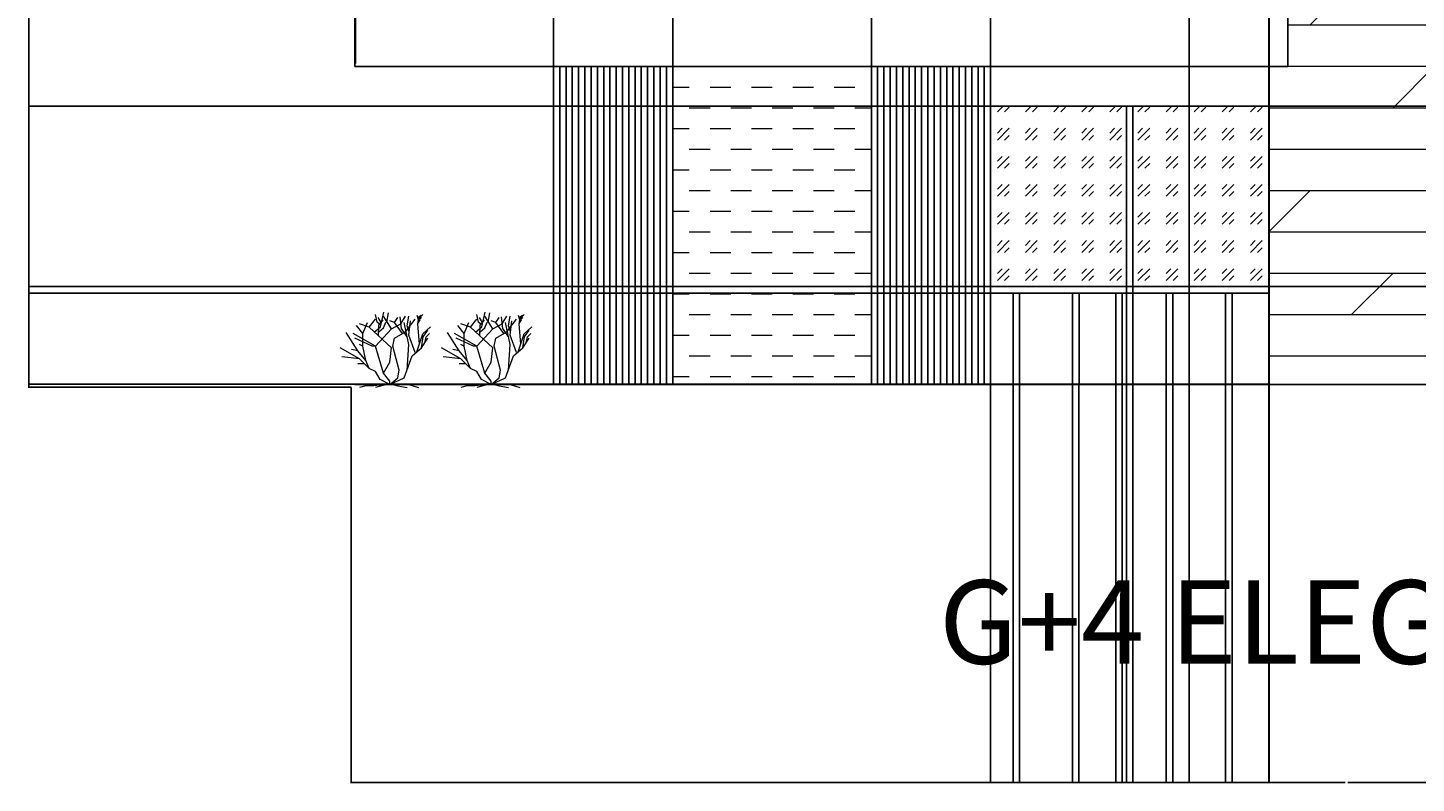
# Model space of a CAD drawing. Units: inches. Extents: x 250 to 1217, y -42 to 832.
# Tile 1 of 7: x 250 to 670, y -42 to 187. Entities that reach past the tile are written whole.
import ezdxf

# ---------------------------------------------------------------- set-up
doc = ezdxf.new("R2010")
doc.units = ezdxf.units.IN
doc.header["$MEASUREMENT"] = 0
for name, color, linetype, lineweight in [('A-ANNO-DIMS', 2, 'Continuous', 18), ('A-ANNO-TEXT', 7, 'Continuous', 25), ('A-ELEV', 7, 'Continuous', 25), ('A-ELEV-PATT', 8, 'Continuous', 13), ('L-PLNT', 3, 'Continuous', 13)]:
    doc.layers.add(name, color=color, linetype=linetype, lineweight=lineweight)
doc.styles.get("Standard").update_dxf_attribs({"font": 'arial.ttf'})
doc.dimstyles.get("Standard").update_dxf_attribs({"dimtxt": 0.18, "dimasz": 0.18, "dimexe": 0.18, "dimexo": 0.0625, "dimgap": 0.09, "dimtad": 0, "dimtih": 1, "dimtoh": 1, "dimdec": 4, "dimzin": 0, "dimdsep": 46, "dimtxsty": 'Standard', "dimcen": 0.09, "dimadec": 0, "dimazin": 0, "dimtfac": 1, "dimtdec": 4, "dimtofl": 0, "dimtmove": 0, "dimatfit": 3, "dimfxl": 1, "dimtolj": 1, "dimtzin": 0, "dimarcsym": 0})

# ---------------------------------------------------------------- blocks, each defined once
blk = doc.blocks.new('*U2')
for p, q in [((-12.471, 19.775), (-12.898, 22.044)), ((-11.28, 19.619), (-12.104, 21.184)), ((-11.433, 18.289), (-10.457, 22.749)), ((-8.16, 17.76), (-10.56, 21.6)), ((-9.48, 19.775), (-8.992, 22.592)), ((-7.2, 19.68), (-6.24, 21.12)), ((-5.086, 17.741), (-5.513, 21.34)), ((-5.28, 19.2), (-3.84, 21.6)), ((-3.377, 18.602), (-2.888, 21.575)), ((-0.508, 21.888), (-0.081, 20.558)), ((-0.203, 19.149), (0.102, 21.34)), ((-0.02, 20.01), (0.896, 21.105)), ((0.041, 20.714), (1.384, 22.044)), ((0.102, 21.34), (0.835, 21.888)), ((-16.8, 16.32), (-18.72, 18.72)), ((-14.88, 18.24), (-17.76, 19.2)), ((-16.8, 16.32), (-15.36, 19.68)), ((-14.88, 18.24), (-12.96, 20.64)), ((-8.16, 12), (-14.88, 18.24)), ((-13.325, 16.724), (-11.433, 18.289)), ((-12.96, 12.48), (-8.16, 17.76)), ((-11.677, 19.071), (-12.471, 19.775)), ((-12.043, 15.628), (-11.921, 18.836)), ((-11.982, 16.802), (-10.579, 18.054)), ((-11.921, 18.836), (-10.64, 20.401)), ((-10.579, 18.054), (-9.846, 19.697)), ((-7.2, 19.68), (-8.64, 20.16)), ((-8.16, 17.76), (-5.28, 19.2)), ((-4.8, 16.32), (-7.2, 19.68)), ((-7.2, 14.88), (-3.84, 16.8)), ((-3.377, 15.315), (-5.086, 17.819)), ((-2.88, 12.96), (-4.32, 19.68)), ((-3.84, 16.8), (-0.96, 20.64)), ((-2.766, 16.802), (-3.377, 18.602)), ((-2.88, 15.84), (-2.4, 20.16)), ((0.346, 13.203), (-0.203, 19.149)), ((-0.142, 19.384), (0.59, 20.401)), ((1.323, 16.254), (3.642, 18.289)), ((1.44, 15.36), (2.88, 17.28)), ((-18.24, 11.04), (-21.755, 16.655)), ((-12.96, 12.48), (-19.68, 16.32)), ((-13.92, 12.48), (-19.2, 14.88)), ((-16.8, 12.48), (-17.76, 12.96)), ((-16.8, 12.48), (-16.8, 16.32)), ((-7.68, 12.48), (-7.2, 14.88)), ((-3.36, 5.28), (-2.88, 12.96)), ((-0.96, 10.56), (-2.88, 15.84)), ((-0.48, 10.8), (0.346, 13.203)), ((0.346, 13.203), (1.323, 16.254)), ((0.96, 12), (1.44, 15.36)), ((0.96, 12), (2.88, 14.88)), ((1.92, 13.44), (2.4, 15.36)), ((2.4, 15.36), (3.36, 16.32)), ((-17.76, 8.64), (-23.663, 11.961)), ((-17.76, 8.64), (-23.128, 9.222)), ((-18.24, 11.04), (-20.16, 11.52)), ((-15.84, 8.16), (-18.24, 11.04)), ((-14.88, 5.76), (-17.76, 8.64)), ((-15.84, 8.16), (-16.8, 12.48)), ((-12.96, 12.48), (-13.92, 12.48)), ((-10.56, 4.32), (-12.96, 12.48)), ((-8.64, 7.68), (-8.16, 12)), ((-6.72, 8.64), (-7.68, 12.48)), ((-5.76, 5.28), (-6.72, 8.64)), ((-4.32, 2.88), (-1.92, 9.6)), ((-1.92, 9.6), (0.96, 12)), ((-16.32, 7.2), (-18.24, 7.2)), ((-14.88, 5.76), (-15.84, 8.16)), ((-12.96, 4.8), (-14.88, 5.76)), ((-11.52, 2.4), (-12.96, 4.8)), ((-10.56, 4.32), (-8.64, 7.68)), ((-8.64, 1.92), (-10.56, 4.32)), ((-6.24, 2.88), (-5.76, 5.28)), ((-15.84, 0.48), (-17.76, 0)), ((-13.44, 0.48), (-15.84, 0.48)), ((-9.6, 0.96), (-13.44, 0.48)), ((-9.6, 0.96), (-12.96, 0)), ((-8.64, 0.96), (-11.52, 2.4)), ((-9.6, 0.96), (-7.68, 0.96)), ((-8.64, 0.96), (-4.32, 2.88)), ((-8.64, 0.96), (-6.24, 2.88)), ((-8.64, 0.96), (-8.64, 1.92)), ((-8.64, 0.96), (-2.88, 0.96)), ((-7.68, 0.96), (-6.24, 0.48)), ((-6.24, 0.48), (-3.36, 0)), ((-2.88, 0.96), (0, 0))]:
    blk.add_line(p, q)
blk = doc.blocks.new('*D7')
at = {"layer": 'A-ANNO-DIMS', "color": 0, "lineweight": -2, "transparency": 16777216}
for p, q in [((347.9, 78), (347.9, -41.6)), ((948.98, 78.86), (948.98, -41.6)), ((348.08, -41.42), (648.06, -41.42)), ((948.8, -41.42), (648.82, -41.42))]:
    blk.add_line(p, q, dxfattribs=at)
at = {"layer": 'A-ANNO-DIMS', "color": 0, "transparency": 16777216}
for points in [[(348.08, -41.39), (348.08, -41.45), (347.9, -41.42)], [(948.8, -41.39), (948.8, -41.45), (948.98, -41.42)]]:
    blk.add_solid(points, dxfattribs=at)
at = {"layer": 'Defpoints', "color": 0, "transparency": 16777216}
for p in [(347.9, 78.06), (948.98, 78.93), (948.98, -41.42)]:
    blk.add_point(p, dxfattribs=at)
at = {"layer": 'A-ANNO-DIMS', "color": 0, "transparency": 16777216, "insert": (648.44, -41.42), "char_height": 0.18, "attachment_point": 5}
blk.add_mtext('\\A1;601.1', dxfattribs=at)
blk = doc.blocks.new('*D11')
at = {"layer": 'A-ANNO-DIMS', "color": 0, "lineweight": -2, "transparency": 16777216}
for p, q in [((352.28, 702.93), (250.36, 702.93)), ((250.54, 702.75), (250.54, 390.68)), ((250.54, 78.24), (250.54, 390.31)), ((347.84, 78.06), (250.36, 78.06))]:
    blk.add_line(p, q, dxfattribs=at)
at = {"layer": 'A-ANNO-DIMS', "color": 0, "transparency": 16777216}
for points in [[(250.51, 702.75), (250.57, 702.75), (250.54, 702.93)], [(250.51, 78.24), (250.57, 78.24), (250.54, 78.06)]]:
    blk.add_solid(points, dxfattribs=at)
at = {"layer": 'Defpoints', "color": 0, "transparency": 16777216}
for p in [(250.54, 702.93), (352.34, 702.93), (347.9, 78.06)]:
    blk.add_point(p, dxfattribs=at)
at = {"layer": 'A-ANNO-DIMS', "color": 0, "transparency": 16777216, "insert": (250.54, 390.49), "char_height": 0.18, "attachment_point": 5}
blk.add_mtext('\\A1;624.9', dxfattribs=at)
blk = doc.blocks.new('*D22')
at = {"layer": 'A-ANNO-DIMS', "color": 0, "lineweight": -2, "transparency": 16777216}
for p, q in [((349.2, 175.91), (349.2, 831.77)), ((349.38, 831.59), (378.7, 831.59)), ((408.8, 831.59), (379.49, 831.59)), ((408.98, 174.99), (408.98, 831.77))]:
    blk.add_line(p, q, dxfattribs=at)
at = {"layer": 'A-ANNO-DIMS', "color": 0, "transparency": 16777216}
for points in [[(349.38, 831.62), (349.38, 831.56), (349.2, 831.59)], [(408.8, 831.62), (408.8, 831.56), (408.98, 831.59)]]:
    blk.add_solid(points, dxfattribs=at)
at = {"layer": 'Defpoints', "color": 0, "transparency": 16777216}
for p in [(408.98, 831.59), (349.2, 175.84), (408.98, 174.93)]:
    blk.add_point(p, dxfattribs=at)
at = {"layer": 'A-ANNO-DIMS', "color": 0, "transparency": 16777216, "insert": (379.09, 831.59), "char_height": 0.18, "attachment_point": 5}
blk.add_mtext('\\A1;59.78', dxfattribs=at)
blk = doc.blocks.new('*D23')
at = {"layer": 'A-ANNO-DIMS', "color": 0, "lineweight": -2, "transparency": 16777216}
for p, q in [((408.98, 174.99), (408.98, 831.77)), ((409.16, 831.59), (426.76, 831.59)), ((444.8, 831.59), (427.2, 831.59)), ((444.98, 174.99), (444.98, 831.77))]:
    blk.add_line(p, q, dxfattribs=at)
at = {"layer": 'A-ANNO-DIMS', "color": 0, "transparency": 16777216}
for points in [[(409.16, 831.62), (409.16, 831.56), (408.98, 831.59)], [(444.8, 831.62), (444.8, 831.56), (444.98, 831.59)]]:
    blk.add_solid(points, dxfattribs=at)
at = {"layer": 'Defpoints', "color": 0, "transparency": 16777216}
for p in [(444.98, 831.59), (408.98, 174.93), (444.98, 174.93)]:
    blk.add_point(p, dxfattribs=at)
at = {"layer": 'A-ANNO-DIMS', "color": 0, "transparency": 16777216, "insert": (426.98, 831.59), "char_height": 0.18, "attachment_point": 5}
blk.add_mtext('\\A1;36', dxfattribs=at)
blk = doc.blocks.new('*D24')
at = {"layer": 'A-ANNO-DIMS', "color": 0, "lineweight": -2, "transparency": 16777216}
for p, q in [((444.98, 174.99), (444.98, 831.77)), ((445.16, 831.59), (474.76, 831.59)), ((504.8, 831.59), (475.2, 831.59)), ((504.98, 174.99), (504.98, 831.77))]:
    blk.add_line(p, q, dxfattribs=at)
at = {"layer": 'A-ANNO-DIMS', "color": 0, "transparency": 16777216}
for points in [[(445.16, 831.62), (445.16, 831.56), (444.98, 831.59)], [(504.8, 831.62), (504.8, 831.56), (504.98, 831.59)]]:
    blk.add_solid(points, dxfattribs=at)
at = {"layer": 'Defpoints', "color": 0, "transparency": 16777216}
for p in [(504.98, 831.59), (444.98, 174.93), (504.98, 174.93)]:
    blk.add_point(p, dxfattribs=at)
at = {"layer": 'A-ANNO-DIMS', "color": 0, "transparency": 16777216, "insert": (474.98, 831.59), "char_height": 0.18, "attachment_point": 5}
blk.add_mtext('\\A1;60', dxfattribs=at)
blk = doc.blocks.new('*D25')
at = {"layer": 'A-ANNO-DIMS', "color": 0, "lineweight": -2, "transparency": 16777216}
for p, q in [((504.98, 174.99), (504.98, 831.77)), ((505.16, 831.59), (522.76, 831.59)), ((540.8, 831.59), (523.2, 831.59)), ((540.98, 174.99), (540.98, 831.77))]:
    blk.add_line(p, q, dxfattribs=at)
at = {"layer": 'A-ANNO-DIMS', "color": 0, "transparency": 16777216}
for points in [[(505.16, 831.62), (505.16, 831.56), (504.98, 831.59)], [(540.8, 831.62), (540.8, 831.56), (540.98, 831.59)]]:
    blk.add_solid(points, dxfattribs=at)
at = {"layer": 'Defpoints', "color": 0, "transparency": 16777216}
for p in [(540.98, 831.59), (504.98, 174.93), (540.98, 174.93)]:
    blk.add_point(p, dxfattribs=at)
at = {"layer": 'A-ANNO-DIMS', "color": 0, "transparency": 16777216, "insert": (522.98, 831.59), "char_height": 0.18, "attachment_point": 5}
blk.add_mtext('\\A1;36', dxfattribs=at)
blk = doc.blocks.new('*D26')
at = {"layer": 'A-ANNO-DIMS', "color": 0, "lineweight": -2, "transparency": 16777216}
for p, q in [((540.98, 174.99), (540.98, 831.77)), ((541.16, 831.59), (582.76, 831.59)), ((624.8, 831.59), (583.2, 831.59)), ((624.98, 174.99), (624.98, 831.77))]:
    blk.add_line(p, q, dxfattribs=at)
at = {"layer": 'A-ANNO-DIMS', "color": 0, "transparency": 16777216}
for points in [[(541.16, 831.62), (541.16, 831.56), (540.98, 831.59)], [(624.8, 831.62), (624.8, 831.56), (624.98, 831.59)]]:
    blk.add_solid(points, dxfattribs=at)
at = {"layer": 'Defpoints', "color": 0, "transparency": 16777216}
for p in [(624.98, 831.59), (540.98, 174.93), (624.98, 174.93)]:
    blk.add_point(p, dxfattribs=at)
at = {"layer": 'A-ANNO-DIMS', "color": 0, "transparency": 16777216, "insert": (582.98, 831.59), "char_height": 0.18, "attachment_point": 5}
blk.add_mtext('\\A1;84', dxfattribs=at)
blk = doc.blocks.new('*D27')
at = {"layer": 'A-ANNO-DIMS', "color": 0, "lineweight": -2, "transparency": 16777216}
for p, q in [((624.98, 174.99), (624.98, 831.77)), ((625.16, 831.59), (655.07, 831.59)), ((685.76, 831.59), (655.86, 831.59)), ((685.94, 176.49), (685.94, 831.77))]:
    blk.add_line(p, q, dxfattribs=at)
at = {"layer": 'A-ANNO-DIMS', "color": 0, "transparency": 16777216}
for points in [[(625.16, 831.62), (625.16, 831.56), (624.98, 831.59)], [(685.76, 831.62), (685.76, 831.56), (685.94, 831.59)]]:
    blk.add_solid(points, dxfattribs=at)
at = {"layer": 'Defpoints', "color": 0, "transparency": 16777216}
for p in [(685.94, 831.59), (685.94, 176.43), (624.98, 174.93)]:
    blk.add_point(p, dxfattribs=at)
at = {"layer": 'A-ANNO-DIMS', "color": 0, "transparency": 16777216, "insert": (655.46, 831.59), "char_height": 0.18, "attachment_point": 5}
blk.add_mtext('\\A1;60.96', dxfattribs=at)
blk = doc.blocks.new('*D35')
at = {"layer": 'A-ANNO-DIMS', "color": 0, "lineweight": -2, "transparency": 16777216}
for p, q in [((624.92, 106.47), (250.36, 106.47)), ((250.54, 106.29), (250.54, 92.88)), ((250.54, 79.11), (250.54, 92.51)), ((624.92, 78.93), (250.36, 78.93))]:
    blk.add_line(p, q, dxfattribs=at)
at = {"layer": 'A-ANNO-DIMS', "color": 0, "transparency": 16777216}
for points in [[(250.51, 106.29), (250.57, 106.29), (250.54, 106.47)], [(250.51, 79.11), (250.57, 79.11), (250.54, 78.93)]]:
    blk.add_solid(points, dxfattribs=at)
at = {"layer": 'Defpoints', "color": 0, "transparency": 16777216}
for p in [(250.54, 106.47), (624.98, 106.47), (624.98, 78.93)]:
    blk.add_point(p, dxfattribs=at)
at = {"layer": 'A-ANNO-DIMS', "color": 0, "transparency": 16777216, "insert": (250.54, 92.7), "char_height": 0.18, "attachment_point": 5}
blk.add_mtext('\\A1;27.54', dxfattribs=at)
blk = doc.blocks.new('*D36')
at = {"layer": 'A-ANNO-DIMS', "color": 0, "lineweight": -2, "transparency": 16777216}
for p, q in [((768.92, 162.93), (250.36, 162.93)), ((250.54, 162.75), (250.54, 135.88)), ((250.54, 108.65), (250.54, 135.51)), ((768.92, 108.47), (250.36, 108.47))]:
    blk.add_line(p, q, dxfattribs=at)
at = {"layer": 'A-ANNO-DIMS', "color": 0, "transparency": 16777216}
for points in [[(250.51, 162.75), (250.57, 162.75), (250.54, 162.93)], [(250.51, 108.65), (250.57, 108.65), (250.54, 108.47)]]:
    blk.add_solid(points, dxfattribs=at)
at = {"layer": 'Defpoints', "color": 0, "transparency": 16777216}
for p in [(250.54, 162.93), (768.98, 162.93), (768.98, 108.47)]:
    blk.add_point(p, dxfattribs=at)
at = {"layer": 'A-ANNO-DIMS', "color": 0, "transparency": 16777216, "insert": (250.54, 135.7), "char_height": 0.18, "attachment_point": 5}
blk.add_mtext('\\A1;54.46', dxfattribs=at)
blk = doc.blocks.new('*D59')
at = {"layer": 'A-ANNO-DIMS', "color": 0, "lineweight": -2, "transparency": 16777216}
for p, q in [((540.98, 78.86), (540.98, -41.6)), ((547.76, 78.86), (547.76, -41.6)), ((541.16, -41.42), (543.98, -41.42)), ((547.58, -41.42), (544.76, -41.42))]:
    blk.add_line(p, q, dxfattribs=at)
at = {"layer": 'A-ANNO-DIMS', "color": 0, "transparency": 16777216}
for points in [[(541.16, -41.39), (541.16, -41.45), (540.98, -41.42)], [(547.58, -41.39), (547.58, -41.45), (547.76, -41.42)]]:
    blk.add_solid(points, dxfattribs=at)
at = {"layer": 'Defpoints', "color": 0, "transparency": 16777216}
for p in [(540.98, 78.93), (547.76, 78.93), (547.76, -41.42)]:
    blk.add_point(p, dxfattribs=at)
at = {"layer": 'A-ANNO-DIMS', "color": 0, "transparency": 16777216, "insert": (544.37, -41.42), "char_height": 0.18, "attachment_point": 5}
blk.add_mtext('\\A1;6.774', dxfattribs=at)
blk = doc.blocks.new('*D60')
at = {"layer": 'A-ANNO-DIMS', "color": 0, "lineweight": -2, "transparency": 16777216}
for p, q in [((549.76, 78.86), (549.76, -41.6)), ((565.68, 78.86), (565.68, -41.6)), ((549.94, -41.42), (557.26, -41.42)), ((565.5, -41.42), (558.18, -41.42))]:
    blk.add_line(p, q, dxfattribs=at)
at = {"layer": 'A-ANNO-DIMS', "color": 0, "transparency": 16777216}
for points in [[(549.94, -41.39), (549.94, -41.45), (549.76, -41.42)], [(565.5, -41.39), (565.5, -41.45), (565.68, -41.42)]]:
    blk.add_solid(points, dxfattribs=at)
at = {"layer": 'Defpoints', "color": 0, "transparency": 16777216}
for p in [(549.76, 78.93), (565.68, 78.93), (565.68, -41.42)]:
    blk.add_point(p, dxfattribs=at)
at = {"layer": 'A-ANNO-DIMS', "color": 0, "transparency": 16777216, "insert": (557.72, -41.42), "char_height": 0.18, "attachment_point": 5}
blk.add_mtext('\\A1;15.928', dxfattribs=at)
blk = doc.blocks.new('*D61')
at = {"layer": 'A-ANNO-DIMS', "color": 0, "lineweight": -2, "transparency": 16777216}
for p, q in [((567.68, 78.86), (567.68, -41.6)), ((578.76, 78.86), (578.76, -41.6)), ((567.86, -41.42), (572.77, -41.42)), ((578.58, -41.42), (573.67, -41.42))]:
    blk.add_line(p, q, dxfattribs=at)
at = {"layer": 'A-ANNO-DIMS', "color": 0, "transparency": 16777216}
for points in [[(567.86, -41.39), (567.86, -41.45), (567.68, -41.42)], [(578.58, -41.39), (578.58, -41.45), (578.76, -41.42)]]:
    blk.add_solid(points, dxfattribs=at)
at = {"layer": 'Defpoints', "color": 0, "transparency": 16777216}
for p in [(567.68, 78.93), (578.76, 78.93), (578.76, -41.42)]:
    blk.add_point(p, dxfattribs=at)
at = {"layer": 'A-ANNO-DIMS', "color": 0, "transparency": 16777216, "insert": (573.22, -41.42), "char_height": 0.18, "attachment_point": 5}
blk.add_mtext('\\A1;11.072', dxfattribs=at)
blk = doc.blocks.new('*D62')
at = {"layer": 'A-ANNO-DIMS', "color": 0, "lineweight": -2, "transparency": 16777216}
for p, q in [((580.76, 78.86), (580.76, -41.6)), ((593.98, 78.86), (593.98, -41.6)), ((580.94, -41.42), (586.91, -41.42)), ((593.8, -41.42), (587.82, -41.42))]:
    blk.add_line(p, q, dxfattribs=at)
at = {"layer": 'A-ANNO-DIMS', "color": 0, "transparency": 16777216}
for points in [[(580.94, -41.39), (580.94, -41.45), (580.76, -41.42)], [(593.8, -41.39), (593.8, -41.45), (593.98, -41.42)]]:
    blk.add_solid(points, dxfattribs=at)
at = {"layer": 'Defpoints', "color": 0, "transparency": 16777216}
for p in [(580.76, 78.93), (593.98, 78.93), (593.98, -41.42)]:
    blk.add_point(p, dxfattribs=at)
at = {"layer": 'A-ANNO-DIMS', "color": 0, "transparency": 16777216, "insert": (587.37, -41.42), "char_height": 0.18, "attachment_point": 5}
blk.add_mtext('\\A1;13.226', dxfattribs=at)
blk = doc.blocks.new('*D63')
at = {"layer": 'A-ANNO-DIMS', "color": 0, "lineweight": -2, "transparency": 16777216}
for p, q in [((595.98, 78.86), (595.98, -41.6)), ((611.91, 78.86), (611.91, -41.6)), ((596.16, -41.42), (603.49, -41.42)), ((611.73, -41.42), (604.4, -41.42))]:
    blk.add_line(p, q, dxfattribs=at)
at = {"layer": 'A-ANNO-DIMS', "color": 0, "transparency": 16777216}
for points in [[(596.16, -41.39), (596.16, -41.45), (595.98, -41.42)], [(611.73, -41.39), (611.73, -41.45), (611.91, -41.42)]]:
    blk.add_solid(points, dxfattribs=at)
at = {"layer": 'Defpoints', "color": 0, "transparency": 16777216}
for p in [(595.98, 78.93), (611.91, 78.93), (611.91, -41.42)]:
    blk.add_point(p, dxfattribs=at)
at = {"layer": 'A-ANNO-DIMS', "color": 0, "transparency": 16777216, "insert": (603.95, -41.42), "char_height": 0.18, "attachment_point": 5}
blk.add_mtext('\\A1;15.928', dxfattribs=at)
blk = doc.blocks.new('*D64')
at = {"layer": 'A-ANNO-DIMS', "color": 0, "lineweight": -2, "transparency": 16777216}
for p, q in [((613.91, 78.86), (613.91, -41.6)), ((624.98, 78.86), (624.98, -41.6)), ((614.09, -41.42), (618.99, -41.42)), ((624.8, -41.42), (619.9, -41.42))]:
    blk.add_line(p, q, dxfattribs=at)
at = {"layer": 'A-ANNO-DIMS', "color": 0, "transparency": 16777216}
for points in [[(614.09, -41.39), (614.09, -41.45), (613.91, -41.42)], [(624.8, -41.39), (624.8, -41.45), (624.98, -41.42)]]:
    blk.add_solid(points, dxfattribs=at)
at = {"layer": 'Defpoints', "color": 0, "transparency": 16777216}
for p in [(613.91, 78.93), (624.98, 78.93), (624.98, -41.42)]:
    blk.add_point(p, dxfattribs=at)
at = {"layer": 'A-ANNO-DIMS', "color": 0, "transparency": 16777216, "insert": (619.45, -41.42), "char_height": 0.18, "attachment_point": 5}
blk.add_mtext('\\A1;11.072', dxfattribs=at)
blk = doc.blocks.new('*D71')
at = {"layer": 'A-ANNO-DIMS', "color": 0, "lineweight": -2, "transparency": 16777216}
for p, q in [((547.76, 106.4), (547.76, -41.6)), ((549.76, 106.4), (549.76, -41.6)), ((547.94, -41.42), (548.43, -41.42)), ((549.58, -41.42), (549.08, -41.42))]:
    blk.add_line(p, q, dxfattribs=at)
at = {"layer": 'A-ANNO-DIMS', "color": 0, "transparency": 16777216}
for points in [[(547.94, -41.39), (547.94, -41.45), (547.76, -41.42)], [(549.58, -41.39), (549.58, -41.45), (549.76, -41.42)]]:
    blk.add_solid(points, dxfattribs=at)
at = {"layer": 'Defpoints', "color": 0, "transparency": 16777216}
for p in [(547.76, 106.47), (549.76, 106.47), (549.76, -41.42)]:
    blk.add_point(p, dxfattribs=at)
at = {"layer": 'A-ANNO-DIMS', "color": 0, "transparency": 16777216, "insert": (548.76, -41.42), "char_height": 0.18, "attachment_point": 5}
blk.add_mtext('\\A1;2.00', dxfattribs=at)
blk = doc.blocks.new('*D72')
at = {"layer": 'A-ANNO-DIMS', "color": 0, "lineweight": -2, "transparency": 16777216}
for p, q in [((540.98, 162.86), (540.98, -41.6)), ((581.98, 162.86), (581.98, -41.6)), ((541.16, -41.42), (561.09, -41.42)), ((581.8, -41.42), (561.88, -41.42))]:
    blk.add_line(p, q, dxfattribs=at)
at = {"layer": 'A-ANNO-DIMS', "color": 0, "transparency": 16777216}
for points in [[(541.16, -41.39), (541.16, -41.45), (540.98, -41.42)], [(581.8, -41.39), (581.8, -41.45), (581.98, -41.42)]]:
    blk.add_solid(points, dxfattribs=at)
at = {"layer": 'Defpoints', "color": 0, "transparency": 16777216}
for p in [(540.98, 162.93), (581.98, 162.93), (581.98, -41.42)]:
    blk.add_point(p, dxfattribs=at)
at = {"layer": 'A-ANNO-DIMS', "color": 0, "transparency": 16777216, "insert": (561.48, -41.42), "char_height": 0.18, "attachment_point": 5}
blk.add_mtext('\\A1;41.00', dxfattribs=at)
blk = doc.blocks.new('*D73')
at = {"layer": 'A-ANNO-DIMS', "color": 0, "lineweight": -2, "transparency": 16777216}
for p, q in [((581.98, 162.86), (581.98, -41.6)), ((583.98, 162.86), (583.98, -41.6)), ((582.16, -41.42), (582.66, -41.42)), ((583.8, -41.42), (583.31, -41.42))]:
    blk.add_line(p, q, dxfattribs=at)
at = {"layer": 'A-ANNO-DIMS', "color": 0, "transparency": 16777216}
for points in [[(582.16, -41.39), (582.16, -41.45), (581.98, -41.42)], [(583.8, -41.39), (583.8, -41.45), (583.98, -41.42)]]:
    blk.add_solid(points, dxfattribs=at)
at = {"layer": 'Defpoints', "color": 0, "transparency": 16777216}
for p in [(581.98, 162.93), (583.98, 162.93), (583.98, -41.42)]:
    blk.add_point(p, dxfattribs=at)
at = {"layer": 'A-ANNO-DIMS', "color": 0, "transparency": 16777216, "insert": (582.98, -41.42), "char_height": 0.18, "attachment_point": 5}
blk.add_mtext('\\A1;2.00', dxfattribs=at)
blk = doc.blocks.new('*D74')
at = {"layer": 'A-ANNO-DIMS', "color": 0, "lineweight": -2, "transparency": 16777216}
for p, q in [((583.98, 162.86), (583.98, -41.6)), ((624.98, 162.86), (624.98, -41.6)), ((584.16, -41.42), (604.09, -41.42)), ((624.8, -41.42), (604.88, -41.42))]:
    blk.add_line(p, q, dxfattribs=at)
at = {"layer": 'A-ANNO-DIMS', "color": 0, "transparency": 16777216}
for points in [[(584.16, -41.39), (584.16, -41.45), (583.98, -41.42)], [(624.8, -41.39), (624.8, -41.45), (624.98, -41.42)]]:
    blk.add_solid(points, dxfattribs=at)
at = {"layer": 'Defpoints', "color": 0, "transparency": 16777216}
for p in [(583.98, 162.93), (624.98, 162.93), (624.98, -41.42)]:
    blk.add_point(p, dxfattribs=at)
at = {"layer": 'A-ANNO-DIMS', "color": 0, "transparency": 16777216, "insert": (604.48, -41.42), "char_height": 0.18, "attachment_point": 5}
blk.add_mtext('\\A1;41.00', dxfattribs=at)
blk = doc.blocks.new('*D95')
at = {"layer": 'A-ANNO-DIMS', "color": 0, "lineweight": -2, "transparency": 16777216}
for p, q in [((625.06, 582.86), (625.06, -41.6)), ((600.97, 582.52), (600.97, -41.6)), ((601.15, -41.42), (612.62, -41.42)), ((624.88, -41.42), (613.41, -41.42))]:
    blk.add_line(p, q, dxfattribs=at)
at = {"layer": 'A-ANNO-DIMS', "color": 0, "transparency": 16777216}
for points in [[(601.15, -41.39), (601.15, -41.45), (600.97, -41.42)], [(624.88, -41.39), (624.88, -41.45), (625.06, -41.42)]]:
    blk.add_solid(points, dxfattribs=at)
at = {"layer": 'Defpoints', "color": 0, "transparency": 16777216}
for p in [(625.06, 582.93), (600.97, 582.58), (625.06, -41.42)]:
    blk.add_point(p, dxfattribs=at)
at = {"layer": 'A-ANNO-DIMS', "color": 0, "transparency": 16777216, "insert": (613.02, -41.42), "char_height": 0.18, "attachment_point": 5}
blk.add_mtext('\\A1;24.10', dxfattribs=at)

msp = doc.modelspace()

# ---------------------------------------------------------------- hatches: boundary and pattern name
at = {"layer": 'A-ELEV-PATT'}
h = msp.add_hatch(dxfattribs=at)
h.set_pattern_fill('DOLMIT', color=256, scale=50)
h.paths.add_polyline_path([(684.9826, 558.9271), (679.1872, 558.9271), (679.1872, 582.9271), (685.0649, 582.9271), (685.0649, 678.9271), (679.1872, 678.9271), (679.1872, 702.9271), (630.7779, 702.9271), (630.7779, 678.9271), (625.0649, 678.9271), (625.0649, 582.9271), (630.7779, 582.9271), (630.7779, 558.9271), (624.9826, 558.9271), (624.9826, 438.9271), (630.7779, 438.9271), (630.7779, 414.9271), (624.9826, 414.9271), (624.9826, 318.9271), (630.7779, 318.9271), (630.7779, 294.9271), (624.9826, 294.9271), (624.9826, 198.9271), (630.7779, 198.9271), (630.7779, 174.9271), (624.9826, 174.9271), (624.9826, 78.9271), (684.9826, 78.9271), (684.9826, 174.9271), (679.1872, 174.9271), (679.1872, 198.9271), (683.6004, 198.9271), (684.9826, 198.9271), (684.9826, 294.9271), (679.1872, 294.9271), (679.1872, 318.9271), (684.9826, 318.9271), (684.9826, 414.9271), (679.1872, 414.9271), (679.1872, 438.9271), (684.9826, 438.9271)])
h = msp.add_hatch(dxfattribs=at)
h.set_pattern_fill('DASH', color=256, scale=50)
h.paths.add_polyline_path([(504.9826, 174.9271), (444.9826, 174.9271), (444.9826, 78.9271), (504.9826, 78.9271)])
h = msp.add_hatch(dxfattribs=at)
h.set_pattern_fill('GOST_GLASS', color=256)
h.set_pattern_definition([(45, (0, 0), (8.48528, 0), [5, -7]), (45, (2.1213, 0), (8.48528, 0), [2, -10]), (45, (0, 2.1213), (8.48528, 0), [2, -10])])
h.paths.add_polyline_path([(581.9826, 162.9271), (540.9826, 162.9271), (540.9826, 108.4651), (578.7563, 108.4651), (581.9826, 108.4651)])
h.paths.add_polyline_path([(624.9826, 162.9271), (583.9826, 162.9271), (583.9826, 108.4651), (624.9826, 108.4651)])

# ---------------------------------------------------------------- linework, layer by layer
at = {"layer": 'A-ELEV'}
for p, q in [((348.9826, 198.9271), (348.9826, 174.9271)), ((630.7779, 198.9271), (630.7779, 174.9271)), ((630.7779, 174.9271), (348.9826, 174.9271)), ((408.9826, 174.9271), (408.9826, 78.9271)), ((410.8773, 174.9271), (410.8773, 78.9271)), ((412.772, 174.9271), (412.772, 78.9271)), ((414.6668, 174.9271), (414.6668, 78.9271)), ((416.5615, 174.9271), (416.5615, 78.9271)), ((418.4563, 174.9271), (418.4563, 78.9271)), ((420.351, 174.9271), (420.351, 78.9271)), ((422.2457, 174.9271), (422.2457, 78.9271)), ((424.1405, 174.9271), (424.1405, 78.9271)), ((426.0352, 174.9271), (426.0352, 78.9271)), ((427.9299, 174.9271), (427.9299, 78.9271)), ((429.8247, 174.9271), (429.8247, 78.9271)), ((431.7194, 174.9271), (431.7194, 78.9271)), ((433.6142, 174.9271), (433.6142, 78.9271)), ((435.5089, 174.9271), (435.5089, 78.9271)), ((437.4036, 174.9271), (437.4036, 78.9271)), ((439.2984, 174.9271), (439.2984, 78.9271)), ((441.1931, 174.9271), (441.1931, 78.9271)), ((443.0878, 174.9271), (443.0878, 78.9271)), ((444.9826, 174.9271), (444.9826, 78.9271)), ((444.9826, 174.9271), (444.9826, 78.9271)), ((444.9826, 174.9271), (444.9826, 78.9271)), ((444.9826, 174.9271), (444.9826, 78.9271)), ((504.9826, 174.9271), (504.9826, 78.9271)), ((506.8773, 174.9271), (506.8773, 78.9271)), ((508.772, 174.9271), (508.772, 78.9271)), ((510.6668, 174.9271), (510.6668, 78.9271)), ((512.5615, 174.9271), (512.5615, 78.9271)), ((514.4563, 174.9271), (514.4563, 78.9271)), ((516.351, 174.9271), (516.351, 78.9271)), ((518.2457, 174.9271), (518.2457, 78.9271)), ((520.1405, 174.9271), (520.1405, 78.9271)), ((522.0352, 174.9271), (522.0352, 78.9271)), ((523.9299, 174.9271), (523.9299, 78.9271)), ((525.8247, 174.9271), (525.8247, 78.9271)), ((527.7194, 174.9271), (527.7194, 78.9271)), ((529.6142, 174.9271), (529.6142, 78.9271)), ((531.5089, 174.9271), (531.5089, 78.9271)), ((533.4036, 174.9271), (533.4036, 78.9271)), ((535.2984, 174.9271), (535.2984, 78.9271)), ((537.1931, 174.9271), (537.1931, 78.9271)), ((539.0878, 174.9271), (539.0878, 78.9271)), ((540.9826, 174.9271), (540.9826, 78.9271)), ((624.9826, 174.9271), (624.9826, 78.9271)), ((540.9826, 162.9271), (624.9826, 162.9271)), ((581.9826, 162.9271), (581.9826, 108.4651)), ((583.9826, 162.9271), (583.9826, 108.4651)), ((578.7563, 108.4651), (540.9826, 108.4651)), ((547.7563, 106.4651), (540.9826, 106.4651)), ((547.7563, 106.4651), (547.7563, 78.9271)), ((549.7563, 106.4651), (549.7563, 78.9271)), ((565.684, 106.4651), (549.7563, 106.4651)), ((624.9826, 108.4651), (564.9826, 108.4651)), ((578.7563, 106.4651), (564.9826, 106.4651)), ((565.684, 106.4651), (565.684, 78.9271)), ((578.7563, 106.4651), (567.684, 106.4651)), ((567.684, 106.4651), (567.684, 78.9271)), ((578.7563, 106.4651), (578.7563, 78.9271)), ((593.9826, 106.4651), (580.7563, 106.4651)), ((580.7563, 106.4651), (580.7563, 78.9271)), ((593.9826, 106.4651), (593.9826, 78.9271)), ((595.9826, 106.4651), (595.9826, 78.9271)), ((611.9103, 106.4651), (595.9826, 106.4651)), ((611.9103, 106.4651), (611.9103, 78.9271)), ((624.9826, 106.4651), (613.9103, 106.4651)), ((613.9103, 106.4651), (613.9103, 78.9271)), ((348.9826, 78.9271), (948.9826, 78.9271))]:
    msp.add_line(p, q, dxfattribs=at)

# ---------------------------------------------------------------- block references
at = {"layer": 'L-PLNT'}
for p in [(368.1829, 77.9671), (398.7837, 77.9671)]:
    msp.add_blockref('*U2', p, dxfattribs=at)

# ---------------------------------------------------------------- texts
at = {"layer": 'A-ANNO-TEXT'}
msp.add_text('G+4 ELEGENT ELEVATION ', height=25.254387, dxfattribs=at).set_placement((525.3922, -5.5103))

# ---------------------------------------------------------------- dimensions: what is measured, and where the dimension line sits
at = {"layer": 'A-ANNO-DIMS'}
for base, p1, p2, override, picture, middle in [((408.9826, 831.5941), (349.204, 175.8442), (408.9826, 174.9271), {"dimdec": 2, "dimlfac": 1, "dimrnd": 0, "dimzin": 0, "dimdsep": 46, "dimlunit": 2}, '*D22', (379.0933, 831.5941)), ((444.9826, 831.5941), (408.9826, 174.9271), (444.9826, 174.9271), {"dimdec": 0, "dimlfac": 1, "dimrnd": 0, "dimzin": 0, "dimdsep": 46, "dimlunit": 2}, '*D23', (426.9826, 831.5941)), ((504.9826, 831.5941), (444.9826, 174.9271), (504.9826, 174.9271), {"dimdec": 0, "dimlfac": 1, "dimrnd": 0, "dimzin": 0, "dimdsep": 46, "dimlunit": 2}, '*D24', (474.9826, 831.5941)), ((540.9826, 831.5941), (504.9826, 174.9271), (540.9826, 174.9271), {"dimdec": 0, "dimlfac": 1, "dimrnd": 0, "dimzin": 0, "dimdsep": 46, "dimlunit": 2}, '*D25', (522.9826, 831.5941)), ((624.9826, 831.5941), (540.9826, 174.9271), (624.9826, 174.9271), {"dimdec": 0, "dimlfac": 1, "dimrnd": 0, "dimzin": 0, "dimdsep": 46, "dimlunit": 2}, '*D26', (582.9826, 831.5941)), ((685.944, 831.5941), (624.9826, 174.9271), (685.944, 176.4321), {"dimdec": 2, "dimlfac": 1, "dimrnd": 0, "dimzin": 0, "dimdsep": 46, "dimlunit": 2}, '*D27', (655.4633, 831.5941)), ((625.0649, -41.4199), (600.9672, 582.5825), (625.0649, 582.9271), {"dimdec": 2, "dimlfac": 1, "dimrnd": 0, "dimzin": 0, "dimdsep": 46, "dimlunit": 2}, '*D95', (613.0161, -41.4199)), ((581.9826, -41.4199), (540.9826, 162.9271), (581.9826, 162.9271), {"dimdec": 2, "dimlfac": 1, "dimrnd": 0, "dimzin": 0, "dimdsep": 46, "dimlunit": 2}, '*D72', (561.4826, -41.4199)), ((583.9826, -41.4199), (581.9826, 162.9271), (583.9826, 162.9271), {"dimdec": 2, "dimlfac": 1, "dimrnd": 0, "dimzin": 0, "dimdsep": 46, "dimlunit": 2}, '*D73', (582.9826, -41.4199)), ((624.9826, -41.4199), (583.9826, 162.9271), (624.9826, 162.9271), {"dimdec": 2, "dimlfac": 1, "dimrnd": 0, "dimzin": 0, "dimdsep": 46, "dimlunit": 2}, '*D74', (604.4826, -41.4199)), ((549.7563, -41.4199), (547.7563, 106.4651), (549.7563, 106.4651), {"dimdec": 2, "dimlfac": 1, "dimrnd": 0, "dimzin": 0, "dimdsep": 46, "dimlunit": 2}, '*D71', (548.7563, -41.4199)), ((948.9826, -41.4199), (347.8976, 78.0612), (948.9826, 78.9271), {"dimdec": 1, "dimlfac": 1, "dimrnd": 0, "dimzin": 0, "dimdsep": 46, "dimlunit": 2}, '*D7', (648.4401, -41.4199)), ((547.7563, -41.4199), (540.9826, 78.9271), (547.7563, 78.9271), {"dimdec": 3, "dimlfac": 1, "dimrnd": 0, "dimzin": 0, "dimdsep": 46, "dimlunit": 2}, '*D59', (544.3694, -41.4199)), ((565.684, -41.4199), (549.7563, 78.9271), (565.684, 78.9271), {"dimdec": 3, "dimlfac": 1, "dimrnd": 0, "dimzin": 0, "dimdsep": 46, "dimlunit": 2}, '*D60', (557.7201, -41.4199)), ((578.7563, -41.4199), (567.684, 78.9271), (578.7563, 78.9271), {"dimdec": 3, "dimlfac": 1, "dimrnd": 0, "dimzin": 0, "dimdsep": 46, "dimlunit": 2}, '*D61', (573.2201, -41.4199)), ((593.9826, -41.4199), (580.7563, 78.9271), (593.9826, 78.9271), {"dimdec": 3, "dimlfac": 1, "dimrnd": 0, "dimzin": 0, "dimdsep": 46, "dimlunit": 2}, '*D62', (587.3694, -41.4199)), ((611.9103, -41.4199), (595.9826, 78.9271), (611.9103, 78.9271), {"dimdec": 3, "dimlfac": 1, "dimrnd": 0, "dimzin": 0, "dimdsep": 46, "dimlunit": 2}, '*D63', (603.9464, -41.4199)), ((624.9826, -41.4199), (613.9103, 78.9271), (624.9826, 78.9271), {"dimdec": 3, "dimlfac": 1, "dimrnd": 0, "dimzin": 0, "dimdsep": 46, "dimlunit": 2}, '*D64', (619.4464, -41.4199))]:
    dim = msp.add_linear_dim(base=base, p1=p1, p2=p2, dimstyle='Standard', override=override, dxfattribs=at)
    dim.commit()
    dim.dimension.update_dxf_attribs({"geometry": picture, "text_midpoint": middle})
for base, p1, p2, override, picture, middle in [((250.5369, 702.9271), (347.8976, 78.0612), (352.3429, 702.9271), {"dimdec": 1, "dimlfac": 1, "dimrnd": 0, "dimzin": 0, "dimdsep": 46, "dimlunit": 2}, '*D11', (250.5369, 390.4941)), ((250.5369, 162.9271), (768.9826, 108.4651), (768.9826, 162.9271), {"dimdec": 2, "dimlfac": 1, "dimrnd": 0, "dimzin": 0, "dimdsep": 46, "dimlunit": 2}, '*D36', (250.5369, 135.6961)), ((250.5369, 106.4651), (624.9826, 78.9271), (624.9826, 106.4651), {"dimdec": 2, "dimlfac": 1, "dimrnd": 0, "dimzin": 0, "dimdsep": 46, "dimlunit": 2}, '*D35', (250.5369, 92.6961))]:
    dim = msp.add_linear_dim(base=base, p1=p1, p2=p2, angle=90, dimstyle='Standard', override=override, dxfattribs=at)
    dim.commit()
    dim.dimension.update_dxf_attribs({"geometry": picture, "text_midpoint": middle})

doc.saveas('drawing.dxf')
